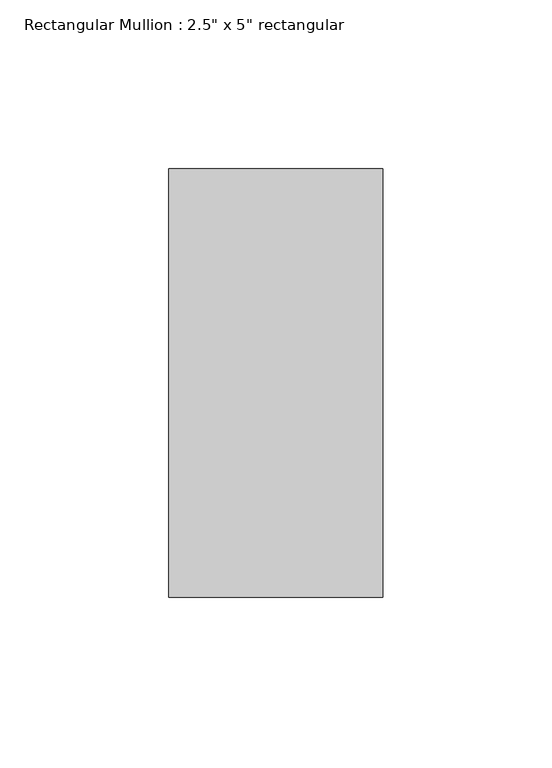
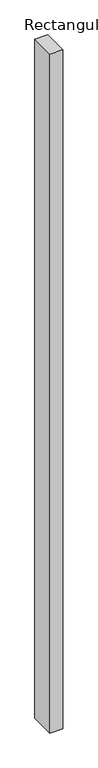
"""IFC4 building model written with IfcOpenShell, lengths in millimetres: member geometry."""

from ifc_helpers import new_model, si_unit, frame, origin, place, context, project, spatial, polyline, outline, extrude, source, transform, mapped, element, save


def member_a8ebf488(model_context):
    return source(origin(), model_context, "Body", "SweptSolid", [
        extrude(outline(polyline([(0.0, 63.5), (0.0, -63.5), (-63.5, -63.5), (-63.5, 63.5), (0.0, 63.5)])), frame((0.0, 0.0, -3506.9820397), z_axis=(0.0, 0.0, 1.0), x_axis=(1.0, 0.0, 0.0)), (0.0, 0.0, 1.0), 3506.9820397),
    ])


if __name__ == "__main__":
    model = new_model("IFC4")
    model_context = context("Model", 3, world=origin())
    ifc_project = project(units=[si_unit("LENGTHUNIT", "METRE", prefix="MILLI")], contexts=[model_context])
    site = spatial("IfcSite", under=ifc_project)
    building = spatial("IfcBuilding", under=site)
    placement = place(None, origin())
    member_shape = member_a8ebf488(model_context)
    element("IfcMember", 1, ObjectType="Rectangular Mullion : 2.5\" x 5\" rectangular", at=placement, inside=building, context=model_context, shape_type="MappedRepresentation", body=[
        mapped(member_shape, transform((0.0, 0.0, 0.0), x_axis=(1.0, 0.0, 0.0), y_axis=(0.0, 1.0, 0.0), z_axis=(0.0, 0.0, 1.0))),
    ])
    save(model, "model.ifc")

# Revit data of these elements
# Type "Rectangular Mullion : 2.5\" x 5\" rectangular"
#   built-in parameter 1007304 = 0.416667 (stored number, unit not read)
#   built-in parameter 1007301 = 0.104167 (stored number, unit not read)
#   built-in parameter 1007300 = 0.104167 (stored number, unit not read)
# Element 1 (IfcMember, "Rectangular Mullion : 2.5\" x 5\" rectangular")
#   Materials on its faces: "Damp-proofing"
# Materials
#   "Damp-proofing": class "Generic", colour RGB 127 127 127, transparency 0, Description = "Damp-proofing", Cost = 0
